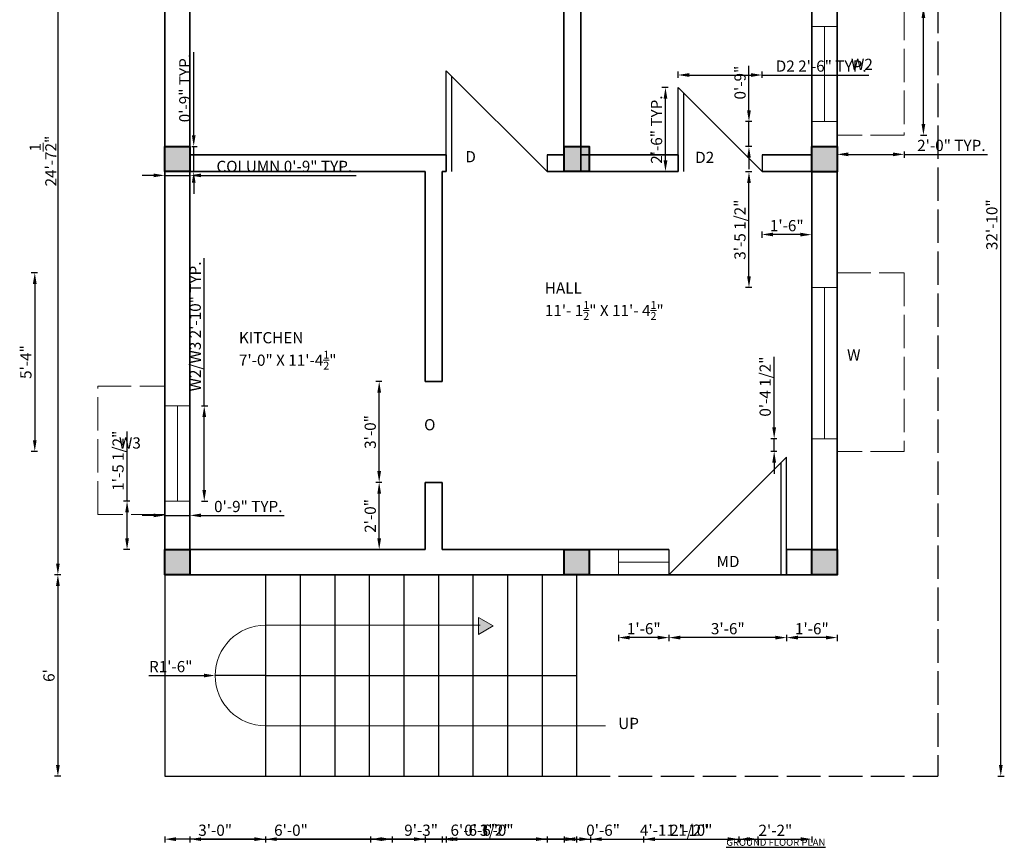
# Model space of a CAD drawing. Units: inches. Extents: x -52 to 299, y -380 to 67.
# Tile 1 of 2: x -52 to 299, y -380 to -84. Entities that reach past the tile are written whole.
import ezdxf

# ---------------------------------------------------------------- set-up
doc = ezdxf.new("R2010")
doc.units = ezdxf.units.IN
doc.linetypes.add('ACAD_ISO02W100', pattern=[15, 12, -3])
for name, color, linetype, lineweight in [('A-ANNO-DIMS', 2, 'Continuous', 18), ('A-ANNO-SYMB', 7, 'Continuous', 18), ('A-ANNO-TEXT', 7, 'Continuous', 18), ('A-ANNO-TITL', 7, 'Continuous', 25), ('A-AREA-IDEN', 7, 'Continuous', 18), ('A-COLS', 7, 'Continuous', 40), ('A-DOOR', 3, 'Continuous', 25), ('A-FLOR-STRS', 7, 'Continuous', 25), ('A-GLAZ', 4, 'Continuous', 18), ('A-ROOF-OVHD', 8, 'ACAD_ISO02W100', 18), ('A-WALL', 7, 'Continuous', 35), ('C-PROP', 8, 'ACAD_ISO02W100', 25)]:
    doc.layers.add(name, color=color, linetype=linetype, lineweight=lineweight)
doc.styles.get("Standard").update_dxf_attribs({"font": 'arial.ttf'})
doc.dimstyles.new('ISO-25', dxfattribs={"dimtxt": 4, "dimasz": 4, "dimexe": 1.25, "dimexo": 0.625, "dimtad": 1, "dimlunit": 4, "dimtxsty": 'Standard', "dimcen": 2.5, "dimadec": 0, "dimazin": 0, "dimtfac": 1, "dimtmove": 0, "dimatfit": 3, "dimfxl": 1, "dimfxlon": 1, "dimarcsym": 0})

# ---------------------------------------------------------------- blocks, each defined once
blk = doc.blocks.new('*D3')
at = {"layer": 'A-ANNO-DIMS', "color": 0, "lineweight": -2, "transparency": 16777216}
for p, q in [((-37.52, 12.8), (-39.77, 12.8)), ((-38.52, 8.8), (-38.52, -278.7)), ((-37.52, -282.7), (-39.77, -282.7))]:
    blk.add_line(p, q, dxfattribs=at)
at = {"layer": 'A-ANNO-DIMS', "color": 0, "transparency": 16777216}
for points in [[(-39.19, 8.8), (-37.85, 8.8), (-38.52, 12.8)], [(-39.19, -278.7), (-37.85, -278.7), (-38.52, -282.7)]]:
    blk.add_solid(points, dxfattribs=at)
at = {"layer": 'Defpoints', "color": 0, "transparency": 16777216}
for p in [(-0.38, 12.8), (-38.52, -282.7), (-0.38, -282.7)]:
    blk.add_point(p, dxfattribs=at)
at = {"layer": 'A-ANNO-DIMS', "color": 0, "transparency": 16777216, "insert": (-43.83, -134.95), "char_height": 4, "attachment_point": 5, "rotation": 90}
blk.add_mtext('24\'-7{\\H1x;\\S1/2;}"', dxfattribs=at)
blk = doc.blocks.new('*D4')
at = {"layer": 'A-ANNO-DIMS', "color": 0, "lineweight": -2, "transparency": 16777216}
for p, q in [((-37.52, -282.7), (-39.77, -282.7)), ((-38.52, -286.7), (-38.52, -350.7)), ((-37.52, -354.7), (-39.77, -354.7))]:
    blk.add_line(p, q, dxfattribs=at)
at = {"layer": 'A-ANNO-DIMS', "color": 0, "transparency": 16777216}
for points in [[(-39.19, -286.7), (-37.86, -286.7), (-38.52, -282.7)], [(-39.19, -350.7), (-37.86, -350.7), (-38.52, -354.7)]]:
    blk.add_solid(points, dxfattribs=at)
at = {"layer": 'Defpoints', "color": 0, "transparency": 16777216}
for p in [(-0.38, -282.7), (-38.52, -354.7), (-0.38, -354.7)]:
    blk.add_point(p, dxfattribs=at)
at = {"layer": 'A-ANNO-DIMS', "color": 0, "transparency": 16777216, "insert": (-41.19, -318.7), "char_height": 4, "attachment_point": 5, "rotation": 90}
blk.add_mtext("6'", dxfattribs=at)
blk = doc.blocks.new('COL-9X9')
h = blk.add_hatch(color=256)
h.dxf.hatch_style = 1
h.paths.add_polyline_path([(0, 0), (9, 0), (9, 9), (0, 9)])
blk.add_lwpolyline([(0, 9), (9, 9), (9, 0), (0, 0)], close=True)
blk = doc.blocks.new('WIN-54')
blk.add_line((0, 4.5), (54, 4.5))
blk.add_lwpolyline([(0, 9), (54, 9), (54, 0), (0, 0)], close=True)
blk = doc.blocks.new('WIN-34')
blk.add_line((4.5, 34), (4.5, 0))
blk.add_lwpolyline([(9, 34), (9, 0), (0, 0), (0, 34)], close=True)
blk = doc.blocks.new('DOOR-D2-30')
for p, q in [((0, 0), (0, 30)), ((30, 0), (0, 30)), ((2, 0), (2, 28)), ((0, 6), (0, 0)), ((30, 6), (30, 0))]:
    blk.add_line(p, q)
blk = doc.blocks.new('WINDOW-SHADE-34')
blk.add_lwpolyline([(0, 45.87), (23.94, 45.87), (23.94, 0), (0, 0)], close=True)
blk = doc.blocks.new('*D10')
at = {"layer": 'A-ANNO-DIMS', "color": 0, "lineweight": -2, "transparency": 16777216}
for p, q in [((-4.38, -140.05), (-8.38, -140.05)), ((-0.38, -139.32), (-0.38, -141.3)), ((-0.38, -140.05), (8.62, -140.05)), ((8.62, -139.32), (8.62, -141.3)), ((12.62, -140.05), (67.98, -140.05))]:
    blk.add_line(p, q, dxfattribs=at)
at = {"layer": 'A-ANNO-DIMS', "color": 0, "transparency": 16777216}
for points in [[(-4.38, -139.38), (-4.38, -140.72), (-0.38, -140.05)], [(12.62, -139.38), (12.62, -140.72), (8.62, -140.05)]]:
    blk.add_solid(points, dxfattribs=at)
at = {"layer": 'Defpoints', "color": 0, "transparency": 16777216}
for p in [(-0.38, -138.7), (8.62, -138.7), (8.62, -140.05)]:
    blk.add_point(p, dxfattribs=at)
at = {"layer": 'A-ANNO-DIMS', "color": 0, "transparency": 16777216, "insert": (42.3, -137.35), "char_height": 4, "attachment_point": 5}
blk.add_mtext('COLUMN 0\'-9" TYP.', dxfattribs=at)
blk = doc.blocks.new('*D11')
at = {"layer": 'A-ANNO-DIMS', "color": 0, "lineweight": -2, "transparency": 16777216}
for p, q in [((9.97, -125.7), (9.97, -96.07)), ((9.25, -129.7), (11.22, -129.7)), ((9.97, -138.7), (9.97, -129.7)), ((9.25, -138.7), (11.22, -138.7)), ((9.97, -142.7), (9.97, -146.7))]:
    blk.add_line(p, q, dxfattribs=at)
at = {"layer": 'A-ANNO-DIMS', "color": 0, "transparency": 16777216}
for points in [[(9.31, -125.7), (10.64, -125.7), (9.97, -129.7)], [(9.31, -142.7), (10.64, -142.7), (9.97, -138.7)]]:
    blk.add_solid(points, dxfattribs=at)
at = {"layer": 'Defpoints', "color": 0, "transparency": 16777216}
for p in [(8.62, -129.7), (9.97, -129.7), (8.62, -138.7)]:
    blk.add_point(p, dxfattribs=at)
at = {"layer": 'A-ANNO-DIMS', "color": 0, "transparency": 16777216, "insert": (7.31, -108.88), "char_height": 4, "attachment_point": 5, "rotation": 90}
blk.add_mtext('0\'-9" TYP.', dxfattribs=at)
blk = doc.blocks.new('*D14')
at = {"layer": 'A-ANNO-DIMS', "color": 0, "lineweight": -2, "transparency": 16777216}
for p, q in [((13.72, -222.4), (13.72, -169.63)), ((12.72, -222.4), (14.97, -222.4)), ((13.72, -252.4), (13.72, -226.4)), ((12.72, -256.4), (14.97, -256.4))]:
    blk.add_line(p, q, dxfattribs=at)
at = {"layer": 'A-ANNO-DIMS', "color": 0, "transparency": 16777216}
for points in [[(13.06, -226.4), (14.39, -226.4), (13.72, -222.4)], [(13.06, -252.4), (14.39, -252.4), (13.72, -256.4)]]:
    blk.add_solid(points, dxfattribs=at)
at = {"layer": 'Defpoints', "color": 0, "transparency": 16777216}
for p in [(8.62, -222.4), (13.72, -222.4), (8.62, -256.4)]:
    blk.add_point(p, dxfattribs=at)
at = {"layer": 'A-ANNO-DIMS', "color": 0, "transparency": 16777216, "insert": (11.03, -194.02), "char_height": 4, "attachment_point": 5, "rotation": 90}
blk.add_mtext('W2/W3 2\'-10" TYP.', dxfattribs=at)
blk = doc.blocks.new('*D15')
at = {"layer": 'A-ANNO-DIMS', "color": 0, "lineweight": -2, "transparency": 16777216}
for p, q in [((-4.38, -261.5), (-8.38, -261.5)), ((-0.38, -260.5), (-0.38, -262.75)), ((-0.38, -261.5), (8.62, -261.5)), ((8.62, -260.5), (8.62, -262.75)), ((12.62, -261.5), (42.25, -261.5))]:
    blk.add_line(p, q, dxfattribs=at)
at = {"layer": 'A-ANNO-DIMS', "color": 0, "transparency": 16777216}
for points in [[(-4.38, -260.84), (-4.38, -262.17), (-0.38, -261.5)], [(12.62, -260.84), (12.62, -262.17), (8.62, -261.5)]]:
    blk.add_solid(points, dxfattribs=at)
at = {"layer": 'Defpoints', "color": 0, "transparency": 16777216}
for p in [(-0.38, -256.4), (8.62, -256.4), (8.62, -261.5)]:
    blk.add_point(p, dxfattribs=at)
at = {"layer": 'A-ANNO-DIMS', "color": 0, "transparency": 16777216, "insert": (29.44, -258.84), "char_height": 4, "attachment_point": 5}
blk.add_mtext('0\'-9" TYP.', dxfattribs=at)
blk = doc.blocks.new('*D16')
at = {"layer": 'A-ANNO-DIMS', "color": 0, "lineweight": -2, "transparency": 16777216}
for p, q in [((182.87, -105.2), (182.87, -102.95)), ((186.87, -104.2), (208.87, -104.2)), ((212.87, -105.2), (212.87, -102.95)), ((212.87, -104.2), (251, -104.2))]:
    blk.add_line(p, q, dxfattribs=at)
at = {"layer": 'A-ANNO-DIMS', "color": 0, "transparency": 16777216}
for points in [[(186.87, -103.53), (186.87, -104.87), (182.87, -104.2)], [(208.87, -103.53), (208.87, -104.87), (212.87, -104.2)]]:
    blk.add_solid(points, dxfattribs=at)
at = {"layer": 'Defpoints', "color": 0, "transparency": 16777216}
for p in [(212.87, -104.2), (182.87, -108.7), (212.87, -108.7)]:
    blk.add_point(p, dxfattribs=at)
at = {"layer": 'A-ANNO-DIMS', "color": 0, "transparency": 16777216, "insert": (233.94, -101.53), "char_height": 4, "attachment_point": 5}
blk.add_mtext('D2 2\'-6" TYP.', dxfattribs=at)
blk = doc.blocks.new('*D17')
at = {"layer": 'A-ANNO-DIMS', "color": 0, "lineweight": -2, "transparency": 16777216}
for p, q in [((179.37, -108.7), (177.12, -108.7)), ((178.37, -134.7), (178.37, -112.7)), ((179.37, -138.7), (177.12, -138.7))]:
    blk.add_line(p, q, dxfattribs=at)
at = {"layer": 'A-ANNO-DIMS', "color": 0, "transparency": 16777216}
for points in [[(177.7, -112.7), (179.04, -112.7), (178.37, -108.7)], [(177.7, -134.7), (179.04, -134.7), (178.37, -138.7)]]:
    blk.add_solid(points, dxfattribs=at)
at = {"layer": 'Defpoints', "color": 0, "transparency": 16777216}
for p in [(178.37, -108.7), (182.87, -108.7), (182.87, -138.7)]:
    blk.add_point(p, dxfattribs=at)
at = {"layer": 'A-ANNO-DIMS', "color": 0, "transparency": 16777216, "insert": (175.7, -123.7), "char_height": 4, "attachment_point": 5, "rotation": 90}
blk.add_mtext('2\'-6" TYP.', dxfattribs=at)
blk = doc.blocks.new('*D18')
at = {"layer": 'A-ANNO-DIMS', "color": 0, "lineweight": -2, "transparency": 16777216}
for p, q in [((270.45, -79.8), (270.45, -0.02)), ((269.45, -79.8), (271.7, -79.8)), ((270.45, -121.66), (270.45, -83.8)), ((269.45, -125.66), (271.7, -125.66))]:
    blk.add_line(p, q, dxfattribs=at)
at = {"layer": 'A-ANNO-DIMS', "color": 0, "transparency": 16777216}
for points in [[(269.78, -83.8), (271.11, -83.8), (270.45, -79.8)], [(269.78, -121.66), (271.11, -121.66), (270.45, -125.66)]]:
    blk.add_solid(points, dxfattribs=at)
at = {"layer": 'Defpoints', "color": 0, "transparency": 16777216}
for p in [(263.57, -79.8), (270.45, -79.8), (263.57, -125.66)]:
    blk.add_point(p, dxfattribs=at)
at = {"layer": 'A-ANNO-DIMS', "color": 0, "transparency": 16777216, "insert": (267.75, -37.91), "char_height": 4, "attachment_point": 5, "rotation": 90}
blk.add_mtext('WINDOW SHADE 3\'-10" TYP.', dxfattribs=at)
blk = doc.blocks.new('*D19')
at = {"layer": 'A-ANNO-DIMS', "color": 0, "lineweight": -2, "transparency": 16777216}
for p, q in [((239.62, -131.54), (239.62, -133.79)), ((243.62, -132.54), (259.57, -132.54)), ((263.57, -131.54), (263.57, -133.79)), ((263.57, -132.54), (293.27, -132.54))]:
    blk.add_line(p, q, dxfattribs=at)
at = {"layer": 'A-ANNO-DIMS', "color": 0, "transparency": 16777216}
for points in [[(243.62, -131.87), (243.62, -133.21), (239.62, -132.54)], [(259.57, -131.87), (259.57, -133.21), (263.57, -132.54)]]:
    blk.add_solid(points, dxfattribs=at)
at = {"layer": 'Defpoints', "color": 0, "transparency": 16777216}
for p in [(239.62, -125.66), (263.57, -125.66), (263.57, -132.54)]:
    blk.add_point(p, dxfattribs=at)
at = {"layer": 'A-ANNO-DIMS', "color": 0, "transparency": 16777216, "insert": (280.42, -129.87), "char_height": 4, "attachment_point": 5}
blk.add_mtext('2\'-0" TYP.', dxfattribs=at)
blk = doc.blocks.new('*D20')
at = {"layer": 'A-ANNO-DIMS', "color": 0, "lineweight": -2, "transparency": 16777216}
for p, q in [((-24.32, 60.81), (-24.32, 63.06)), ((-20.32, 61.81), (271.62, 61.81)), ((275.62, 60.81), (275.62, 63.06))]:
    blk.add_line(p, q, dxfattribs=at)
at = {"layer": 'A-ANNO-DIMS', "color": 0, "transparency": 16777216}
for points in [[(-20.32, 62.47), (-20.32, 61.14), (-24.32, 61.81)], [(271.62, 62.47), (271.62, 61.14), (275.62, 61.81)]]:
    blk.add_solid(points, dxfattribs=at)
at = {"layer": 'Defpoints', "color": 0, "transparency": 16777216}
for p in [(275.62, 61.81), (275.62, 12.8), (-24.32, -215.36)]:
    blk.add_point(p, dxfattribs=at)
at = {"layer": 'A-ANNO-DIMS', "color": 0, "transparency": 16777216, "insert": (125.65, 64.47), "char_height": 4, "attachment_point": 5}
blk.add_mtext('25\'-0"', dxfattribs=at)
blk = doc.blocks.new('*D21')
at = {"layer": 'A-ANNO-DIMS', "color": 0, "lineweight": -2, "transparency": 16777216}
for p, q in [((297.07, 39.36), (299.32, 39.36)), ((298.07, -350.7), (298.07, 35.36)), ((297.07, -354.7), (299.32, -354.7))]:
    blk.add_line(p, q, dxfattribs=at)
at = {"layer": 'A-ANNO-DIMS', "color": 0, "transparency": 16777216}
for points in [[(297.41, 35.36), (298.74, 35.36), (298.07, 39.36)], [(297.41, -350.7), (298.74, -350.7), (298.07, -354.7)]]:
    blk.add_solid(points, dxfattribs=at)
at = {"layer": 'Defpoints', "color": 0, "transparency": 16777216}
for p in [(151.63, 39.36), (298.07, 39.36), (275.62, -354.7)]:
    blk.add_point(p, dxfattribs=at)
at = {"layer": 'A-ANNO-DIMS', "color": 0, "transparency": 16777216, "insert": (295.4, -157.67), "char_height": 4, "attachment_point": 5, "rotation": 90}
blk.add_mtext('32\'-10"', dxfattribs=at)
blk = doc.blocks.new('*D22')
at = {"layer": 'A-ANNO-DIMS', "color": 0, "lineweight": -2, "transparency": 16777216}
for p, q in [((35.62, -376.15), (35.62, -378.4)), ((142.66, -377.15), (39.62, -377.15)), ((146.66, -376.15), (146.66, -378.4))]:
    blk.add_line(p, q, dxfattribs=at)
at = {"layer": 'A-ANNO-DIMS', "color": 0, "transparency": 16777216}
for points in [[(39.62, -376.48), (39.62, -377.82), (35.62, -377.15)], [(142.66, -376.48), (142.66, -377.82), (146.66, -377.15)]]:
    blk.add_solid(points, dxfattribs=at)
at = {"layer": 'Defpoints', "color": 0, "transparency": 16777216}
for p in [(35.62, -354.7), (146.66, -354.7), (35.62, -377.15)]:
    blk.add_point(p, dxfattribs=at)
at = {"layer": 'A-ANNO-DIMS', "color": 0, "transparency": 16777216, "insert": (91.14, -374.48), "char_height": 4, "attachment_point": 5}
blk.add_mtext('9\'-3"', dxfattribs=at)
blk = doc.blocks.new('*D23')
at = {"layer": 'A-ANNO-DIMS', "color": 0, "lineweight": -2, "transparency": 16777216}
for p, q in [((-0.38, -376.15), (-0.38, -378.4)), ((31.62, -377.15), (3.62, -377.15)), ((35.62, -376.15), (35.62, -378.4))]:
    blk.add_line(p, q, dxfattribs=at)
at = {"layer": 'A-ANNO-DIMS', "color": 0, "transparency": 16777216}
for points in [[(3.62, -376.48), (3.62, -377.82), (-0.38, -377.15)], [(31.62, -376.48), (31.62, -377.82), (35.62, -377.15)]]:
    blk.add_solid(points, dxfattribs=at)
at = {"layer": 'Defpoints', "color": 0, "transparency": 16777216}
for p in [(-0.38, -354.7), (35.62, -354.7), (-0.38, -377.15)]:
    blk.add_point(p, dxfattribs=at)
at = {"layer": 'A-ANNO-DIMS', "color": 0, "transparency": 16777216, "insert": (17.62, -374.48), "char_height": 4, "attachment_point": 5}
blk.add_mtext('3\'-0"', dxfattribs=at)
blk = doc.blocks.new('*D24')
at = {"layer": 'A-ANNO-DIMS', "color": 0, "lineweight": -2, "transparency": 16777216}
for p, q in [((8.62, -376.15), (8.62, -378.4)), ((12.62, -377.15), (76.75, -377.15)), ((80.75, -376.15), (80.75, -378.4))]:
    blk.add_line(p, q, dxfattribs=at)
at = {"layer": 'A-ANNO-DIMS', "color": 0, "transparency": 16777216}
for points in [[(12.62, -376.48), (12.62, -377.82), (8.62, -377.15)], [(76.75, -376.48), (76.75, -377.82), (80.75, -377.15)]]:
    blk.add_solid(points, dxfattribs=at)
at = {"layer": 'Defpoints', "color": 0, "transparency": 16777216}
for p in [(8.62, 3.8), (80.75, 3.8), (80.75, -377.15)]:
    blk.add_point(p, dxfattribs=at)
at = {"layer": 'A-ANNO-DIMS', "color": 0, "transparency": 16777216, "insert": (44.69, -374.48), "char_height": 4, "attachment_point": 5}
blk.add_mtext('6\'-0"', dxfattribs=at)
blk = doc.blocks.new('*D25')
at = {"layer": 'A-ANNO-DIMS', "color": 0, "lineweight": -2, "transparency": 16777216}
for p, q in [((170.58, -376.15), (170.58, -378.4)), ((174.58, -377.15), (200.58, -377.15)), ((204.58, -376.15), (204.58, -378.4))]:
    blk.add_line(p, q, dxfattribs=at)
at = {"layer": 'A-ANNO-DIMS', "color": 0, "transparency": 16777216}
for points in [[(174.58, -376.48), (174.58, -377.82), (170.58, -377.15)], [(200.58, -376.48), (200.58, -377.82), (204.58, -377.15)]]:
    blk.add_solid(points, dxfattribs=at)
at = {"layer": 'Defpoints', "color": 0, "transparency": 16777216}
for p in [(170.58, 3.8), (204.58, 3.8), (204.58, -377.15)]:
    blk.add_point(p, dxfattribs=at)
at = {"layer": 'A-ANNO-DIMS', "color": 0, "transparency": 16777216, "insert": (187.58, -374.48), "char_height": 4, "attachment_point": 5}
blk.add_mtext('2\'-10"', dxfattribs=at)
blk = doc.blocks.new('*D26')
at = {"layer": 'A-ANNO-DIMS', "color": 0, "lineweight": -2, "transparency": 16777216}
for p, q in [((204.58, -376.15), (204.58, -378.4)), ((208.58, -377.15), (226.62, -377.15)), ((230.62, -376.15), (230.62, -378.4))]:
    blk.add_line(p, q, dxfattribs=at)
at = {"layer": 'A-ANNO-DIMS', "color": 0, "transparency": 16777216}
for points in [[(208.58, -376.48), (208.58, -377.82), (204.58, -377.15)], [(226.62, -376.48), (226.62, -377.82), (230.62, -377.15)]]:
    blk.add_solid(points, dxfattribs=at)
at = {"layer": 'Defpoints', "color": 0, "transparency": 16777216}
for p in [(204.58, 3.8), (230.62, 3.8), (230.62, -377.15)]:
    blk.add_point(p, dxfattribs=at)
at = {"layer": 'A-ANNO-DIMS', "color": 0, "transparency": 16777216, "insert": (217.6, -374.52), "char_height": 4, "attachment_point": 5}
blk.add_mtext('2\'-2"', dxfattribs=at)
blk = doc.blocks.new('*D27')
at = {"layer": 'A-ANNO-DIMS', "color": 0, "lineweight": -2, "transparency": 16777216}
for p, q in [((208.17, -116.86), (208.17, -100.98)), ((209.17, -120.86), (206.92, -120.86)), ((208.17, -129.78), (208.17, -120.86)), ((209.17, -129.78), (206.92, -129.78)), ((208.17, -133.78), (208.17, -137.78))]:
    blk.add_line(p, q, dxfattribs=at)
at = {"layer": 'A-ANNO-DIMS', "color": 0, "transparency": 16777216}
for points in [[(207.51, -116.86), (208.84, -116.86), (208.17, -120.86)], [(207.51, -133.78), (208.84, -133.78), (208.17, -129.78)]]:
    blk.add_solid(points, dxfattribs=at)
at = {"layer": 'Defpoints', "color": 0, "transparency": 16777216}
for p in [(208.17, -120.86), (230.62, -120.86), (230.62, -129.78)]:
    blk.add_point(p, dxfattribs=at)
at = {"layer": 'A-ANNO-DIMS', "color": 0, "transparency": 16777216, "insert": (205.51, -106.92), "char_height": 4, "attachment_point": 5, "rotation": 90}
blk.add_mtext('0\'-9"', dxfattribs=at)
blk = doc.blocks.new('*D28')
at = {"layer": 'A-ANNO-DIMS', "color": 0, "lineweight": -2, "transparency": 16777216}
for p, q in [((209.17, -138.78), (206.92, -138.78)), ((208.17, -176.1), (208.17, -142.78)), ((209.17, -180.1), (206.92, -180.1))]:
    blk.add_line(p, q, dxfattribs=at)
at = {"layer": 'A-ANNO-DIMS', "color": 0, "transparency": 16777216}
for points in [[(207.51, -142.78), (208.84, -142.78), (208.17, -138.78)], [(207.51, -176.1), (208.84, -176.1), (208.17, -180.1)]]:
    blk.add_solid(points, dxfattribs=at)
at = {"layer": 'Defpoints', "color": 0, "transparency": 16777216}
for p in [(208.17, -138.78), (230.62, -138.78), (230.62, -180.1)]:
    blk.add_point(p, dxfattribs=at)
at = {"layer": 'A-ANNO-DIMS', "color": 0, "transparency": 16777216, "insert": (205.48, -159.44), "char_height": 4, "attachment_point": 5, "rotation": 90}
blk.add_mtext('3\'-5 1/2"', dxfattribs=at)
blk = doc.blocks.new('*D29')
at = {"layer": 'A-ANNO-DIMS', "color": 0, "lineweight": -2, "transparency": 16777216}
for p, q in [((-13.83, -256.4), (-13.82, -231.57)), ((-12.83, -256.4), (-15.08, -256.4)), ((-13.83, -269.7), (-13.83, -260.4)), ((-12.83, -273.7), (-15.08, -273.69))]:
    blk.add_line(p, q, dxfattribs=at)
at = {"layer": 'A-ANNO-DIMS', "color": 0, "transparency": 16777216}
for points in [[(-14.49, -260.4), (-13.16, -260.4), (-13.83, -256.4)], [(-14.5, -269.7), (-13.16, -269.7), (-13.83, -273.7)]]:
    blk.add_solid(points, dxfattribs=at)
at = {"layer": 'Defpoints', "color": 0, "transparency": 16777216}
for p in [(-13.83, -256.4), (8.62, -256.4), (8.62, -273.7)]:
    blk.add_point(p, dxfattribs=at)
at = {"layer": 'A-ANNO-DIMS', "color": 0, "transparency": 16777216, "insert": (-16.52, -241.98), "char_height": 4, "attachment_point": 5, "rotation": 89.9896}
blk.add_mtext('1\'-5 1/2"', dxfattribs=at)
blk = doc.blocks.new('*D30')
at = {"layer": 'A-ANNO-DIMS', "color": 0, "lineweight": -2, "transparency": 16777216}
for p, q in [((179.62, -304.15), (179.62, -306.4)), ((217.62, -305.15), (183.62, -305.15)), ((221.62, -304.15), (221.62, -306.4))]:
    blk.add_line(p, q, dxfattribs=at)
at = {"layer": 'A-ANNO-DIMS', "color": 0, "transparency": 16777216}
for points in [[(183.62, -304.48), (183.62, -305.82), (179.62, -305.15)], [(217.62, -304.48), (217.62, -305.82), (221.62, -305.15)]]:
    blk.add_solid(points, dxfattribs=at)
at = {"layer": 'Defpoints', "color": 0, "transparency": 16777216}
for p in [(179.62, -282.7), (221.62, -282.7), (179.62, -305.15)]:
    blk.add_point(p, dxfattribs=at)
at = {"layer": 'A-ANNO-DIMS', "color": 0, "transparency": 16777216, "insert": (200.62, -302.48), "char_height": 4, "attachment_point": 5}
blk.add_mtext('3\'-6"', dxfattribs=at)
blk = doc.blocks.new('*D31')
at = {"layer": 'A-ANNO-DIMS', "color": 0, "lineweight": -2, "transparency": 16777216}
for p, q in [((221.62, -304.15), (221.62, -306.4)), ((235.62, -305.15), (225.62, -305.15)), ((239.62, -304.15), (239.62, -306.4))]:
    blk.add_line(p, q, dxfattribs=at)
at = {"layer": 'A-ANNO-DIMS', "color": 0, "transparency": 16777216}
for points in [[(225.62, -304.48), (225.62, -305.82), (221.62, -305.15)], [(235.62, -304.48), (235.62, -305.82), (239.62, -305.15)]]:
    blk.add_solid(points, dxfattribs=at)
at = {"layer": 'Defpoints', "color": 0, "transparency": 16777216}
for p in [(221.62, -282.7), (239.62, -282.7), (221.62, -305.15)]:
    blk.add_point(p, dxfattribs=at)
at = {"layer": 'A-ANNO-DIMS', "color": 0, "transparency": 16777216, "insert": (230.62, -302.48), "char_height": 4, "attachment_point": 5}
blk.add_mtext('1\'-6"', dxfattribs=at)
blk = doc.blocks.new('*D32')
at = {"layer": 'A-ANNO-DIMS', "color": 0, "lineweight": -2, "transparency": 16777216}
for p, q in [((161.62, -304.15), (161.62, -306.4)), ((175.62, -305.15), (165.62, -305.15)), ((179.62, -304.15), (179.62, -306.4))]:
    blk.add_line(p, q, dxfattribs=at)
at = {"layer": 'A-ANNO-DIMS', "color": 0, "transparency": 16777216}
for points in [[(165.62, -304.48), (165.62, -305.82), (161.62, -305.15)], [(175.62, -304.48), (175.62, -305.82), (179.62, -305.15)]]:
    blk.add_solid(points, dxfattribs=at)
at = {"layer": 'Defpoints', "color": 0, "transparency": 16777216}
for p in [(161.62, -282.7), (179.62, -282.7), (161.62, -305.15)]:
    blk.add_point(p, dxfattribs=at)
at = {"layer": 'A-ANNO-DIMS', "color": 0, "transparency": 16777216, "insert": (170.62, -302.48), "char_height": 4, "attachment_point": 5}
blk.add_mtext('1\'-6"', dxfattribs=at)
blk = doc.blocks.new('*D33')
at = {"layer": 'A-ANNO-DIMS', "color": 0, "lineweight": -2, "transparency": 16777216}
for p, q in [((100.12, -376.15), (100.12, -378.4)), ((104.12, -377.15), (132.12, -377.15)), ((136.12, -376.15), (136.12, -378.4))]:
    blk.add_line(p, q, dxfattribs=at)
at = {"layer": 'A-ANNO-DIMS', "color": 0, "transparency": 16777216}
for points in [[(104.12, -376.48), (104.12, -377.82), (100.12, -377.15)], [(132.12, -376.48), (132.12, -377.82), (136.12, -377.15)]]:
    blk.add_solid(points, dxfattribs=at)
at = {"layer": 'Defpoints', "color": 0, "transparency": 16777216}
for p in [(100.12, -138.7), (136.12, -138.7), (136.12, -377.15)]:
    blk.add_point(p, dxfattribs=at)
at = {"layer": 'A-ANNO-DIMS', "color": 0, "transparency": 16777216, "insert": (118.12, -374.48), "char_height": 4, "attachment_point": 5}
blk.add_mtext('3\'-0"', dxfattribs=at)
blk = doc.blocks.new('*D34')
at = {"layer": 'A-ANNO-DIMS', "color": 0, "lineweight": -2, "transparency": 16777216}
for p, q in [((132.12, -377.15), (128.12, -377.15)), ((136.12, -376.15), (136.12, -378.4)), ((136.12, -377.15), (142.15, -377.15)), ((142.15, -376.15), (142.15, -378.4)), ((146.15, -377.15), (162.04, -377.15))]:
    blk.add_line(p, q, dxfattribs=at)
at = {"layer": 'A-ANNO-DIMS', "color": 0, "transparency": 16777216}
for points in [[(132.12, -376.48), (132.12, -377.82), (136.12, -377.15)], [(146.15, -376.48), (146.15, -377.82), (142.15, -377.15)]]:
    blk.add_solid(points, dxfattribs=at)
at = {"layer": 'Defpoints', "color": 0, "transparency": 16777216}
for p in [(136.12, -138.7), (142.15, -138.7), (142.15, -377.15)]:
    blk.add_point(p, dxfattribs=at)
at = {"layer": 'A-ANNO-DIMS', "color": 0, "transparency": 16777216, "insert": (156.1, -374.48), "char_height": 4, "attachment_point": 5}
blk.add_mtext('0\'-6"', dxfattribs=at)
blk = doc.blocks.new('*D35')
at = {"layer": 'A-ANNO-DIMS', "color": 0, "lineweight": -2, "transparency": 16777216}
for p, q in [((212.78, -160.15), (212.77, -162.4)), ((226.53, -161.21), (216.77, -161.17)), ((230.53, -160.23), (230.52, -162.48))]:
    blk.add_line(p, q, dxfattribs=at)
at = {"layer": 'A-ANNO-DIMS', "color": 0, "transparency": 16777216}
for points in [[(216.78, -160.5), (216.77, -161.83), (212.77, -161.15)], [(226.53, -160.54), (226.52, -161.88), (230.53, -161.23)]]:
    blk.add_solid(points, dxfattribs=at)
at = {"layer": 'Defpoints', "color": 0, "transparency": 16777216}
for p in [(212.87, -138.7), (230.62, -138.78), (212.77, -161.15)]:
    blk.add_point(p, dxfattribs=at)
at = {"layer": 'A-ANNO-DIMS', "color": 0, "transparency": 16777216, "insert": (221.66, -158.52), "char_height": 4, "attachment_point": 5, "rotation": 359.7528}
blk.add_mtext('1\'-6"', dxfattribs=at)
blk = doc.blocks.new('*D37')
at = {"layer": 'A-ANNO-DIMS', "color": 0, "lineweight": -2, "transparency": 16777216}
for p, q in [((77.17, -213.7), (74.92, -213.7)), ((76.17, -245.7), (76.17, -217.7)), ((77.17, -249.7), (74.92, -249.7))]:
    blk.add_line(p, q, dxfattribs=at)
at = {"layer": 'A-ANNO-DIMS', "color": 0, "transparency": 16777216}
for points in [[(75.51, -217.7), (76.84, -217.7), (76.17, -213.7)], [(75.51, -245.7), (76.84, -245.7), (76.17, -249.7)]]:
    blk.add_solid(points, dxfattribs=at)
at = {"layer": 'Defpoints', "color": 0, "transparency": 16777216}
for p in [(76.17, -213.7), (98.62, -213.7), (98.62, -249.7)]:
    blk.add_point(p, dxfattribs=at)
at = {"layer": 'A-ANNO-DIMS', "color": 0, "transparency": 16777216, "insert": (73.5, -231.7), "char_height": 4, "attachment_point": 5, "rotation": 90}
blk.add_mtext('3\'-0"', dxfattribs=at)
blk = doc.blocks.new('*D38')
at = {"layer": 'A-ANNO-DIMS', "color": 0, "lineweight": -2, "transparency": 16777216}
for p, q in [((77.17, -249.7), (74.92, -249.7)), ((76.17, -269.7), (76.17, -253.7)), ((77.17, -273.7), (74.92, -273.7))]:
    blk.add_line(p, q, dxfattribs=at)
at = {"layer": 'A-ANNO-DIMS', "color": 0, "transparency": 16777216}
for points in [[(75.51, -253.7), (76.84, -253.7), (76.17, -249.7)], [(75.51, -269.7), (76.84, -269.7), (76.17, -273.7)]]:
    blk.add_solid(points, dxfattribs=at)
at = {"layer": 'Defpoints', "color": 0, "transparency": 16777216}
for p in [(76.17, -249.7), (98.62, -249.7), (98.62, -273.7)]:
    blk.add_point(p, dxfattribs=at)
at = {"layer": 'A-ANNO-DIMS', "color": 0, "transparency": 16777216, "insert": (73.51, -261.7), "char_height": 4, "attachment_point": 5, "rotation": 90}
blk.add_mtext('2\'-0"', dxfattribs=at)
blk = doc.blocks.new('*D39')
at = {"layer": 'A-ANNO-DIMS', "color": 0, "lineweight": -2, "transparency": 16777216}
for p, q in [((88.62, -377.15), (84.62, -377.15)), ((92.62, -376.15), (92.62, -378.4)), ((92.62, -377.15), (98.62, -377.15)), ((98.62, -376.15), (98.62, -378.4)), ((102.62, -377.15), (118.51, -377.15))]:
    blk.add_line(p, q, dxfattribs=at)
at = {"layer": 'A-ANNO-DIMS', "color": 0, "transparency": 16777216}
for points in [[(88.62, -376.48), (88.62, -377.82), (92.62, -377.15)], [(102.62, -376.48), (102.62, -377.82), (98.62, -377.15)]]:
    blk.add_solid(points, dxfattribs=at)
at = {"layer": 'Defpoints', "color": 0, "transparency": 16777216}
for p in [(92.62, -213.7), (98.62, -213.7), (98.62, -377.15)]:
    blk.add_point(p, dxfattribs=at)
at = {"layer": 'A-ANNO-DIMS', "color": 0, "transparency": 16777216, "insert": (112.56, -374.48), "char_height": 4, "attachment_point": 5}
blk.add_mtext('0\'-6"', dxfattribs=at)
blk = doc.blocks.new('*D42')
at = {"layer": 'A-ANNO-DIMS', "color": 0, "lineweight": -2, "transparency": 16777216}
for p, q in [((73.09, -376.15), (73.09, -378.4)), ((77.09, -377.15), (147.63, -377.15)), ((151.63, -376.15), (151.63, -378.4))]:
    blk.add_line(p, q, dxfattribs=at)
at = {"layer": 'A-ANNO-DIMS', "color": 0, "transparency": 16777216}
for points in [[(77.09, -376.48), (77.09, -377.82), (73.09, -377.15)], [(147.63, -376.48), (147.63, -377.82), (151.63, -377.15)]]:
    blk.add_solid(points, dxfattribs=at)
at = {"layer": 'Defpoints', "color": 0, "transparency": 16777216}
for p in [(73.09, 39.36), (151.63, 39.36), (151.63, -377.15)]:
    blk.add_point(p, dxfattribs=at)
at = {"layer": 'A-ANNO-DIMS', "color": 0, "transparency": 16777216, "insert": (112.36, -374.46), "char_height": 4, "attachment_point": 5}
blk.add_mtext('6\'-6 1/2"', dxfattribs=at)
blk = doc.blocks.new('*D43')
at = {"layer": 'A-ANNO-DIMS', "color": 0, "lineweight": -2, "transparency": 16777216}
for p, q in [((151.63, -376.15), (151.63, -378.4)), ((155.63, -377.15), (207.36, -377.15)), ((211.36, -376.15), (211.36, -378.4))]:
    blk.add_line(p, q, dxfattribs=at)
at = {"layer": 'A-ANNO-DIMS', "color": 0, "transparency": 16777216}
for points in [[(155.63, -376.48), (155.63, -377.82), (151.63, -377.15)], [(207.36, -376.48), (207.36, -377.82), (211.36, -377.15)]]:
    blk.add_solid(points, dxfattribs=at)
at = {"layer": 'Defpoints', "color": 0, "transparency": 16777216}
for p in [(151.63, 27.28), (211.36, 27.28), (211.36, -377.15)]:
    blk.add_point(p, dxfattribs=at)
at = {"layer": 'A-ANNO-DIMS', "color": 0, "transparency": 16777216, "insert": (181.49, -374.46), "char_height": 4, "attachment_point": 5}
blk.add_mtext('4\'-11 1/2"', dxfattribs=at)
blk = doc.blocks.new('*D44')
at = {"layer": 'A-ANNO-DIMS', "color": 0, "lineweight": -2, "transparency": 16777216}
for p, q in [((-45.77, -174.82), (-48.02, -174.82)), ((-46.77, -178.82), (-46.77, -234.64)), ((-45.77, -238.64), (-48.02, -238.64))]:
    blk.add_line(p, q, dxfattribs=at)
at = {"layer": 'A-ANNO-DIMS', "color": 0, "transparency": 16777216}
for points in [[(-47.44, -178.82), (-46.1, -178.82), (-46.77, -174.82)], [(-47.44, -234.64), (-46.1, -234.64), (-46.77, -238.64)]]:
    blk.add_solid(points, dxfattribs=at)
at = {"layer": 'Defpoints', "color": 0, "transparency": 16777216}
for p in [(263.57, -174.82), (-46.77, -238.64), (263.57, -238.64)]:
    blk.add_point(p, dxfattribs=at)
at = {"layer": 'A-ANNO-DIMS', "color": 0, "transparency": 16777216, "insert": (-49.43, -206.73), "char_height": 4, "attachment_point": 5, "rotation": 90}
blk.add_mtext('5\'-4"', dxfattribs=at)
blk = doc.blocks.new('*D45')
at = {"layer": 'A-ANNO-DIMS', "color": 0, "lineweight": -2, "transparency": 16777216}
for p, q in [((217.17, -230.1), (217.17, -204.9)), ((218.17, -234.1), (215.92, -234.1)), ((217.17, -238.64), (217.17, -234.1)), ((218.17, -238.64), (215.92, -238.64)), ((217.17, -242.64), (217.17, -246.64))]:
    blk.add_line(p, q, dxfattribs=at)
at = {"layer": 'A-ANNO-DIMS', "color": 0, "transparency": 16777216}
for points in [[(216.51, -230.1), (217.84, -230.1), (217.17, -234.1)], [(216.51, -242.64), (217.84, -242.64), (217.17, -238.64)]]:
    blk.add_solid(points, dxfattribs=at)
at = {"layer": 'Defpoints', "color": 0, "transparency": 16777216}
for p in [(217.17, -234.1), (239.62, -234.1), (239.62, -238.64)]:
    blk.add_point(p, dxfattribs=at)
at = {"layer": 'A-ANNO-DIMS', "color": 0, "transparency": 16777216, "insert": (214.48, -215.5), "char_height": 4, "attachment_point": 5, "rotation": 90}
blk.add_mtext('0\'-4 1/2"', dxfattribs=at)
blk = doc.blocks.new('*D46')
at = {"layer": 'A-ANNO-DIMS', "color": 0, "lineweight": -2, "transparency": 16777216}
for p, q in [((-6.09, -318.7), (13.62, -318.7)), ((35.62, -318.7), (17.62, -318.7))]:
    blk.add_line(p, q, dxfattribs=at)
at = {"layer": 'A-ANNO-DIMS', "color": 0, "transparency": 16777216}
blk.add_solid([(13.62, -318.03), (13.62, -319.37), (17.62, -318.7)], dxfattribs=at)
at = {"layer": 'Defpoints', "color": 0, "transparency": 16777216}
for p in [(17.62, -318.7), (35.62, -318.7)]:
    blk.add_point(p, dxfattribs=at)
at = {"layer": 'A-ANNO-DIMS', "color": 0, "transparency": 16777216, "insert": (1.76, -316.03), "char_height": 4, "attachment_point": 5, "rotation": 359.9991}
blk.add_mtext('R1\'-6"', dxfattribs=at)

msp = doc.modelspace()

# ---------------------------------------------------------------- hatches: boundary and pattern name
at = {"layer": 'A-ANNO-SYMB'}
h = msp.add_hatch(color=256, dxfattribs=at)
h.dxf.hatch_style = 1
h.paths.add_polyline_path([(116.83, -300.986), (111.634, -297.986), (111.634, -303.986)])

# ---------------------------------------------------------------- linework, layer by layer
for p, q in [((35.62, -300.699), (112.249, -300.699)), ((146.656, -336.699), (35.62, -336.699)), ((146.656, -336.699), (157.014, -336.699))]:
    msp.add_line(p, q, dxfattribs=at)
msp.add_lwpolyline([(111.634, -297.986), (111.634, -303.986), (116.83, -300.986)], close=True, dxfattribs=at)
msp.add_arc((35.62, -318.699), 18, 90, 270, dxfattribs=at)
at = {"layer": 'A-DOOR'}
for p, q in [((100.123, -138.699), (100.123, -102.699)), ((136.123, -138.699), (100.123, -102.699)), ((102.123, -138.699), (102.123, -104.699)), ((100.123, -132.699), (100.123, -138.699)), ((136.123, -132.699), (136.123, -138.699)), ((179.623, -282.699), (221.623, -240.699)), ((221.623, -282.699), (221.623, -240.699)), ((219.623, -282.699), (219.623, -242.699)), ((179.623, -273.699), (179.623, -282.699)), ((221.623, -273.699), (221.623, -282.699))]:
    msp.add_line(p, q, dxfattribs=at)
at = {"layer": 'A-FLOR-STRS'}
for p, q in [((-0.38, -282.699), (-0.38, -354.699)), ((35.62, -282.699), (35.62, -354.699)), ((47.957, -282.699), (47.957, -354.699)), ((60.295, -282.699), (60.295, -354.699)), ((72.632, -282.699), (72.632, -354.699)), ((84.969, -282.699), (84.969, -354.699)), ((97.307, -282.699), (97.307, -354.699)), ((109.644, -282.699), (109.644, -354.699)), ((121.982, -282.699), (121.982, -354.699)), ((134.319, -282.699), (134.319, -354.699)), ((146.656, -282.699), (146.656, -354.699)), ((146.656, -282.699), (146.656, -354.699)), ((35.62, -318.699), (146.656, -318.699)), ((-0.38, -354.699), (146.656, -354.699))]:
    msp.add_line(p, q, dxfattribs=at)
at = {"layer": 'A-GLAZ'}
for p, q in [((161.623, -273.699), (161.623, -282.699)), ((161.623, -278.199), (179.623, -278.199))]:
    msp.add_line(p, q, dxfattribs=at)
at = {"layer": 'A-ROOF-OVHD'}
msp.add_lwpolyline([(239.623, -174.824), (263.567, -174.824), (263.567, -238.636), (239.623, -238.636)], close=True, dxfattribs=at)
at = {"layer": 'A-WALL'}
for p, q in [((-0.377, -282.699), (-0.377, 12.801)), ((239.623, 12.801), (239.623, -282.699)), ((8.623, -273.699), (8.623, 3.801)), ((142.123, -138.699), (142.123, -38.199)), ((148.123, -138.699), (148.123, -50.199)), ((230.623, -50.199), (230.623, -273.699)), ((8.623, -132.699), (100.123, -132.699)), ((136.123, -132.699), (142.123, -132.699)), ((148.123, -132.699), (182.871, -132.699)), ((212.871, -132.699), (230.623, -132.699)), ((8.623, -138.699), (92.623, -138.699)), ((92.623, -138.699), (92.623, -213.699)), ((98.623, -138.699), (98.623, -213.699)), ((98.623, -138.699), (100.123, -138.699)), ((136.123, -138.699), (142.123, -138.699)), ((148.123, -138.699), (182.871, -138.699)), ((212.871, -138.699), (230.623, -138.699)), ((98.623, -213.699), (92.623, -213.699)), ((98.623, -249.699), (92.623, -249.699)), ((92.623, -249.699), (92.623, -273.699)), ((98.623, -249.699), (98.623, -273.699)), ((92.623, -273.699), (8.623, -273.699)), ((179.623, -273.699), (98.623, -273.699)), ((230.623, -273.699), (221.623, -273.699)), ((239.623, -282.699), (-0.377, -282.699))]:
    msp.add_line(p, q, dxfattribs=at)
at = {"layer": 'C-PROP'}
for p in [(275.623, 12.801), (146.656, -354.699)]:
    msp.add_line(p, (275.623, -354.699), dxfattribs=at)

# ---------------------------------------------------------------- block references
at = {"layer": 'A-COLS'}
for p in [(-0.377, -138.699), (142.154, -138.699), (230.623, -138.776), (-0.38, -282.699), (142.156, -282.699), (230.623, -282.699)]:
    msp.add_blockref('COL-9X9', p, dxfattribs=at)
at = {"layer": 'A-DOOR'}
msp.add_blockref('DOOR-D2-30', (182.871, -138.699), dxfattribs=at)
at = {"layer": 'A-GLAZ'}
for p in [(230.623, -120.863), (-0.377, -256.403)]:
    msp.add_blockref('WIN-34', p, dxfattribs=at)
at = {"layer": 'A-GLAZ', "rotation": 270}
msp.add_blockref('WIN-54', (230.623, -180.105), dxfattribs=at)
at = {"layer": 'A-ROOF-OVHD'}
for p in [(239.623, -125.661), (-24.321, -261.222)]:
    msp.add_blockref('WINDOW-SHADE-34', p, dxfattribs=at)

# ---------------------------------------------------------------- texts
at = {"layer": 'A-ANNO-TEXT', "char_height": 4, "attachment_point": 1}
for s, width, insert in [('W2', 9.80024, (244.583, -98.398)), ('D', 17.12441, (106.937, -131.378)), ('D2', 9.84438, (188.982, -131.624)), ('W', 9.37912, (243.189, -202.175)), ('O', 6.88677, (92.204, -227.117)), ('W3', 10.5538, (-16.725, -233.632)), ('MD', 9.37078, (196.61, -275.947)), ('UP', 13.2205, (161.509, -333.81))]:
    msp.add_mtext_dynamic_manual_height_columns(s, width=width, gutter_width=12.5, heights=[0], dxfattribs=dict(at, insert=insert))
at = {"layer": 'A-ANNO-TITL', "insert": (200.089, -377.023), "char_height": 2.5, "attachment_point": 1}
msp.add_mtext_dynamic_manual_height_columns('{\\fArial|b1|i0|c0|p34;\\LGROUND FLOOR PLAN}', width=160.71292, gutter_width=12.5, heights=[0], dxfattribs=at)
at = {"layer": 'A-AREA-IDEN', "char_height": 4, "attachment_point": 1}
for s, width, insert in [('\\A1;HALL\\P11\'- 1{\\H0.7x;\\S1/2;}" X 11\'- 4{\\H0.7x;\\S1/2;}"', 62.40107, (135.309, -178.276)), ('\\A1;KITCHEN\\P7\'-0" X 11\'-4{\\H0.7x;\\S1/2;}"', 42.62904, (26.104, -196.04))]:
    msp.add_mtext_dynamic_manual_height_columns(s, width=width, gutter_width=12.5, heights=[0], dxfattribs=dict(at, insert=insert))

# ---------------------------------------------------------------- dimensions: what is measured, and where the dimension line sits
at = {"layer": 'A-ANNO-DIMS'}
for base, p1, p2, picture, middle in [((275.623, 61.807), (-24.321, -215.357), (275.623, 12.801), '*D20', (125.651, 64.474)), ((151.625, -377.149), (73.092, 39.357), (151.625, 39.357), '*D42', (112.359, -374.456)), ((211.364, -377.149), (151.625, 27.284), (211.364, 27.284), '*D43', (181.495, -374.456)), ((80.748, -377.149), (8.623, 3.801), (80.748, 3.801), '*D24', (44.686, -374.482)), ((204.585, -377.149), (170.585, 3.801), (204.585, 3.801), '*D25', (187.585, -374.482)), ((230.623, -377.149), (204.585, 3.801), (230.623, 3.801), '*D26', (217.604, -374.516)), ((136.123, -377.149), (100.123, -138.699), (136.123, -138.699), '*D33', (118.123, -374.481)), ((142.154, -377.149), (136.123, -138.699), (142.154, -138.699), '*D34', (156.095, -374.482)), ((98.623, -377.149), (92.623, -213.699), (98.623, -213.699), '*D39', (112.564, -374.482))]:
    dim = msp.add_linear_dim(base=base, p1=p1, p2=p2, dimstyle='ISO-25', override={"dimdec": 1, "dimlfac": 1, "dimrnd": 0, "dimzin": 1, "dimdsep": 46, "dimlunit": 4, "dimfrac": 2}, dxfattribs=at)
    dim.commit()
    dim.dimension.update_dxf_attribs({"geometry": picture, "text_midpoint": middle})
for base, p1, p2, angle, override, picture, middle in [((298.073, 39.357), (275.623, -354.699), (151.625, 39.357), 90, {"dimdec": 1, "dimlfac": 1, "dimrnd": 0, "dimzin": 1, "dimdsep": 46, "dimlunit": 4, "dimfrac": 2}, '*D21', (295.404, -157.671)), ((-38.52, -282.699), (-0.377, 12.801), (-0.38, -282.699), 90, {"dimclrd": 0, "dimclre": 0, "dimclrt": 0}, '*D3', (-43.828, -134.949)), ((208.173, -120.863), (230.623, -129.776), (230.623, -120.863), 90, {"dimdec": 1, "dimlfac": 1, "dimrnd": 0, "dimzin": 1, "dimdsep": 46, "dimlunit": 4, "dimfrac": 2}, '*D27', (205.506, -106.921)), ((208.173, -138.776), (230.623, -180.105), (230.623, -138.776), 90, {"dimdec": 1, "dimlfac": 1, "dimrnd": 0, "dimzin": 1, "dimdsep": 46, "dimlunit": 4, "dimfrac": 2}, '*D28', (205.478, -159.44)), ((212.775, -161.149), (230.623, -138.776), (212.871, -138.699), 179.75277, {"dimdec": 1, "dimlfac": 1, "dimrnd": 0, "dimzin": 1, "dimdsep": 46, "dimlunit": 4, "dimfrac": 2}, '*D35', (221.662, -158.52)), ((-46.771, -238.636), (263.567, -174.824), (263.567, -238.636), 90, {"dimdec": 1, "dimlfac": 1, "dimrnd": 0, "dimzin": 1, "dimdsep": 46, "dimlunit": 4, "dimfrac": 2}, '*D44', (-49.43, -206.73)), ((217.173, -234.105), (239.623, -238.636), (239.623, -234.105), 90, {"dimdec": 1, "dimlfac": 1, "dimrnd": 0, "dimzin": 1, "dimdsep": 46, "dimlunit": 4, "dimfrac": 2}, '*D45', (214.48, -215.503)), ((76.173, -213.699), (98.623, -249.699), (98.623, -213.699), 90, {"dimdec": 1, "dimlfac": 1, "dimrnd": 0, "dimzin": 1, "dimdsep": 46, "dimlunit": 4, "dimfrac": 2}, '*D37', (73.504, -231.699)), ((-13.827, -256.399), (8.62, -273.699), (8.623, -256.403), 89.98958, {"dimdec": 1, "dimlfac": 1, "dimrnd": 0, "dimzin": 1, "dimdsep": 46, "dimlunit": 4, "dimfrac": 2}, '*D29', (-16.518, -241.985)), ((76.173, -249.699), (98.623, -273.699), (98.623, -249.699), 90, {"dimdec": 1, "dimlfac": 1, "dimrnd": 0, "dimzin": 1, "dimdsep": 46, "dimlunit": 4, "dimfrac": 2}, '*D38', (73.506, -261.699)), ((-38.522, -354.699), (-0.38, -282.699), (-0.38, -354.699), 90, {"dimclrd": 0, "dimclre": 0, "dimclrt": 0}, '*D4', (-41.189, -318.699)), ((161.623, -305.149), (179.623, -282.699), (161.623, -282.699), 180, {"dimdec": 1, "dimlfac": 1, "dimrnd": 0, "dimzin": 1, "dimdsep": 46, "dimlunit": 4, "dimfrac": 2}, '*D32', (170.623, -302.482)), ((179.623, -305.149), (221.623, -282.699), (179.623, -282.699), 180, {"dimdec": 1, "dimlfac": 1, "dimrnd": 0, "dimzin": 1, "dimdsep": 46, "dimlunit": 4, "dimfrac": 2}, '*D30', (200.623, -302.481)), ((221.623, -305.149), (239.623, -282.699), (221.623, -282.699), 180, {"dimdec": 1, "dimlfac": 1, "dimrnd": 0, "dimzin": 1, "dimdsep": 46, "dimlunit": 4, "dimfrac": 2}, '*D31', (230.623, -302.482)), ((-0.38, -377.149), (35.62, -354.699), (-0.38, -354.699), 180, {"dimdec": 1, "dimlfac": 1, "dimrnd": 0, "dimzin": 1, "dimdsep": 46, "dimlunit": 4, "dimfrac": 2}, '*D23', (17.62, -374.481)), ((35.62, -377.149), (146.656, -354.699), (35.62, -354.699), 180, {"dimdec": 1, "dimlfac": 1, "dimrnd": 0, "dimzin": 1, "dimdsep": 46, "dimlunit": 4, "dimfrac": 2}, '*D22', (91.138, -374.481))]:
    dim = msp.add_linear_dim(base=base, p1=p1, p2=p2, angle=angle, dimstyle='ISO-25', override=override, dxfattribs=at)
    dim.commit()
    dim.dimension.update_dxf_attribs({"geometry": picture, "text_midpoint": middle})
for base, p1, p2, text, picture, middle in [((270.447, -79.796), (263.567, -125.661), (263.567, -79.796), 'WINDOW SHADE <> TYP.', '*D18', (267.751, -37.906)), ((9.973, -129.699), (8.623, -138.699), (8.623, -129.699), '<> TYP.', '*D11', (7.306, -108.883)), ((178.371, -108.699), (182.871, -138.699), (182.871, -108.699), '<> TYP.', '*D17', (175.704, -123.699)), ((13.723, -222.403), (8.623, -256.403), (8.623, -222.403), 'W2/W3 <> TYP.', '*D14', (11.028, -194.017))]:
    dim = msp.add_linear_dim(base=base, p1=p1, p2=p2, angle=90, text=text, dimstyle='ISO-25', override={"dimdec": 1, "dimlfac": 1, "dimrnd": 0, "dimzin": 1, "dimdsep": 46, "dimlunit": 4, "dimfrac": 2}, dxfattribs=at)
    dim.commit()
    dim.dimension.update_dxf_attribs({"geometry": picture, "text_midpoint": middle})
for base, p1, p2, text, picture, middle in [((212.871, -104.199), (182.871, -108.699), (212.871, -108.699), 'D2 <> TYP.', '*D16', (233.936, -101.532)), ((263.567, -132.541), (239.623, -125.661), (263.567, -125.661), '<> TYP.', '*D19', (280.417, -129.873)), ((8.623, -140.049), (-0.377, -138.699), (8.623, -138.699), 'COLUMN <> TYP.', '*D10', (42.3, -137.355)), ((8.623, -261.503), (-0.377, -256.403), (8.623, -256.403), '<> TYP.', '*D15', (29.439, -258.836))]:
    dim = msp.add_linear_dim(base=base, p1=p1, p2=p2, text=text, dimstyle='ISO-25', override={"dimdec": 1, "dimlfac": 1, "dimrnd": 0, "dimzin": 1, "dimdsep": 46, "dimlunit": 4, "dimfrac": 2}, dxfattribs=at)
    dim.commit()
    dim.dimension.update_dxf_attribs({"geometry": picture, "text_midpoint": middle})
dim = msp.add_radius_dim(center=(35.62, -318.699), mpoint=(17.62, -318.699), dimstyle='ISO-25', override={"dimdec": 1, "dimlfac": 1, "dimrnd": 0, "dimzin": 1, "dimdsep": 46, "dimlunit": 4, "dimfrac": 2}, dxfattribs=at)
dim.commit()
dim.dimension.update_dxf_attribs({"geometry": '*D46', "text_midpoint": (1.764, -316.031)})

doc.saveas('drawing.dxf')
